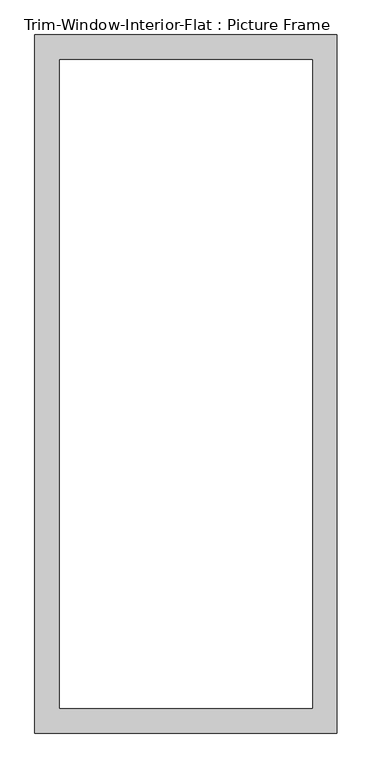
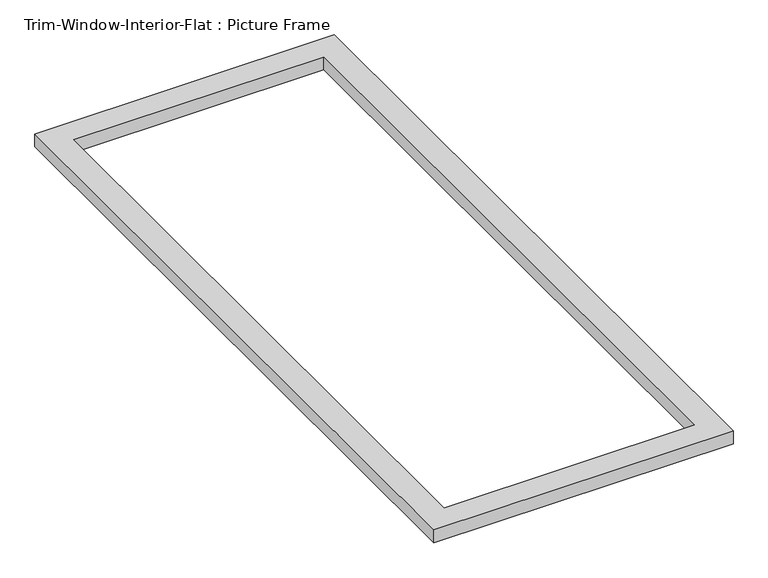
"""IFC4 building model written with IfcOpenShell, lengths in millimetres: proxy geometry, Trim-Window-Interior-Flat : Picture Frame."""

from ifc_helpers import new_model, si_unit, origin, origin_with_axes, place, context, project, spatial, polyline, outline, extrude, source, transform, mapped, element, save


def trim_window_interior_flat_picture_frame_978fd00d(model_context):
    return source(origin(), model_context, "Body", "SweptSolid", [
        extrude(outline(polyline([(349.25, 44.45), (349.25, -1568.45), (-349.25, -1568.45), (-349.25, 44.45), (349.25, 44.45)]), holes=[polyline([(292.1, -12.7), (-292.1, -12.7), (-292.1, -1511.3), (292.1, -1511.3), (292.1, -12.7)])]), origin_with_axes(), (0.0, 0.0, 1.0), 31.75),
    ])


if __name__ == "__main__":
    model = new_model("IFC4")
    model_context = context("Model", 3, world=origin())
    ifc_project = project(units=[si_unit("LENGTHUNIT", "METRE", prefix="MILLI")], contexts=[model_context])
    site = spatial("IfcSite", under=ifc_project)
    building = spatial("IfcBuilding", under=site)
    placement = place(None, origin())
    trim_window_interior_flat_picture_frame_shape = trim_window_interior_flat_picture_frame_978fd00d(model_context)
    element("IfcBuildingElementProxy", 1, Name="Trim-Window-Interior-Flat : Picture Frame", ObjectType="Trim-Window-Interior-Flat : Picture Frame", at=placement, inside=building, context=model_context, shape_type="MappedRepresentation", body=[
        mapped(trim_window_interior_flat_picture_frame_shape, transform((0.0, 0.0, 0.0), x_axis=(1.0, 0.0, 0.0), y_axis=(0.0, 1.0, 0.0), z_axis=(0.0, 0.0, 1.0))),
    ])
    save(model, "model.ifc")

# Revit data of these elements
# Type "Trim-Window-Interior-Flat : Picture Frame"
#   Trim Thickness_Picture Frame = 0' - 1 1/4"
#   Trim Width = 0' - 2 1/4"
#   Trim Thickness_with Sill = 0' - 0 3/4"
#   Sill Thickness = 0' - 1 1/4"
#   Opening Width [instance default] = 2' - 0"
#   Opening Height [instance default] = 3' - 0"
#   Default Elevation = 4' - 0"
#   Sill = no
#   Picture Frame = yes
#   Trim Material [instance default] = none
# Element 1 (IfcBuildingElementProxy, "Trim-Window-Interior-Flat : Picture Frame")
#   Opening Height = 5' - 0"
#   Trim Material = Wood - Stained
#   Materials on its faces: "Wood - Stained"
# Materials
#   "Wood - Stained": class "Wood", colour RGB 224 178 126, transparency 0, Cost = 0
